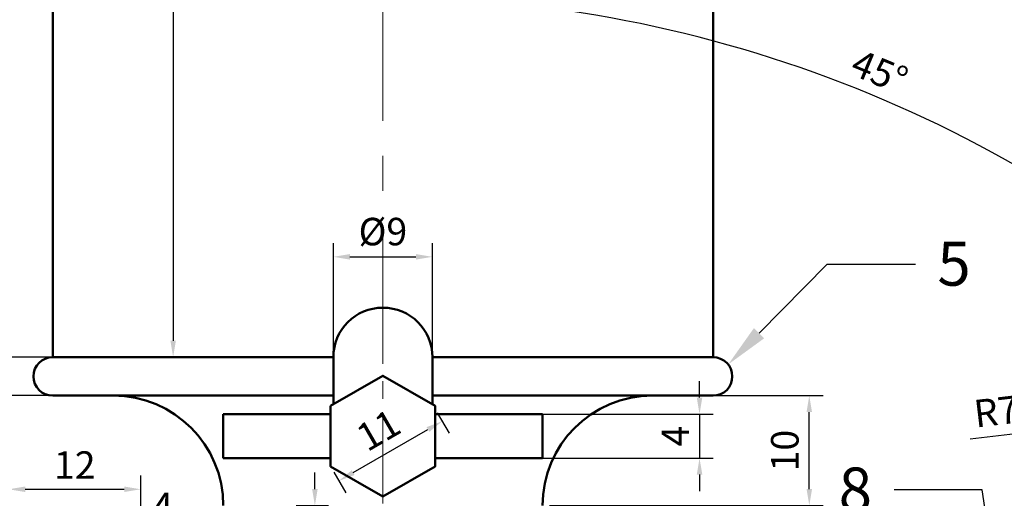
# Model space of a CAD drawing. Units: millimetres. Extents: x -414 to 17, y 81 to 417.
# Tile 4 of 7: x -341 to -252, y 214 to 257. Entities that reach past the tile are written whole.
import ezdxf
from ezdxf import colors
from ezdxf.entities.mleader import LeaderData, LeaderLine
from ezdxf.math import Vec2, Vec3

# ---------------------------------------------------------------- set-up
doc = ezdxf.new("R2010")
doc.units = ezdxf.units.MM
doc.header["$LTSCALE"] = 0.5
doc.linetypes.add('CENTER', pattern=[50.8, 31.75, -6.35, 6.35, -6.35])
for name, color, linetype, lineweight in [('M-CNTR', 1, 'CENTER', 18), ('M-DIMS', 2, 'Continuous', 25), ('M-OUTL', 7, 'Continuous', 50)]:
    doc.layers.add(name, color=color, linetype=linetype, lineweight=lineweight)
doc.styles.get("Standard").update_dxf_attribs({"font": 'arial.ttf'})
doc.dimstyles.new('ISO-25', dxfattribs={"dimtxt": 2.5, "dimasz": 1.5, "dimexe": 1.25, "dimexo": 0.625, "dimtad": 1, "dimtoh": 1, "dimdec": 0, "dimtxsty": 'Standard', "dimcen": 2.5, "dimadec": 0, "dimazin": 0, "dimtfac": 1, "dimtdec": 0, "dimtmove": 0, "dimatfit": 3, "dimfxl": 1, "dimarcsym": 0})

# ---------------------------------------------------------------- blocks, each defined once
blk = doc.blocks.new('*D18')
at = {"layer": 'Defpoints', "color": 0, "ltscale": 0.5, "transparency": 16777216}
for p in [(-328.257, 299.461), (-328.257, 226.461), (-327.548, 226.461)]:
    blk.add_point(p, dxfattribs=at)
at = {"layer": 'M-DIMS', "color": 0, "lineweight": -2, "ltscale": 0.5, "transparency": 16777216}
for p, q in [((-327.632, 299.461), (-326.298, 299.461)), ((-327.548, 297.961), (-327.548, 227.961)), ((-327.632, 226.461), (-326.298, 226.461))]:
    blk.add_line(p, q, dxfattribs=at)
at = {"layer": 'M-DIMS', "color": 0, "ltscale": 0.5, "transparency": 16777216}
for points in [[(-327.798, 297.961), (-327.298, 297.961), (-327.548, 299.461)], [(-327.798, 227.961), (-327.298, 227.961), (-327.548, 226.461)]]:
    blk.add_solid(points, dxfattribs=at)
at = {"layer": 'M-DIMS', "color": 0, "ltscale": 0.5, "transparency": 16777216, "insert": (-329.45, 262.961), "char_height": 2.5, "attachment_point": 5, "rotation": 90}
blk.add_mtext('73', dxfattribs=at)
blk = doc.blocks.new('*D19')
at = {"layer": 'Defpoints', "color": 0, "ltscale": 0.5, "transparency": 16777216}
for p in [(-303.993, 235.587), (-312.993, 226.461), (-303.993, 226.461)]:
    blk.add_point(p, dxfattribs=at)
at = {"layer": 'M-DIMS', "color": 0, "lineweight": -2, "ltscale": 0.5, "transparency": 16777216}
for p, q in [((-312.993, 227.086), (-312.993, 236.837)), ((-303.993, 227.086), (-303.993, 236.837)), ((-311.493, 235.587), (-305.493, 235.587))]:
    blk.add_line(p, q, dxfattribs=at)
at = {"layer": 'M-DIMS', "color": 0, "ltscale": 0.5, "transparency": 16777216}
for points in [[(-311.493, 235.837), (-311.493, 235.337), (-312.993, 235.587)], [(-305.493, 235.837), (-305.493, 235.337), (-303.993, 235.587)]]:
    blk.add_solid(points, dxfattribs=at)
at = {"layer": 'M-DIMS', "color": 0, "ltscale": 0.5, "transparency": 16777216, "insert": (-308.493, 237.559), "char_height": 2.5, "attachment_point": 5}
blk.add_mtext('%%C9', dxfattribs=at)
blk = doc.blocks.new('*D20')
at = {"layer": 'Defpoints', "color": 0, "ltscale": 0.5, "transparency": 16777216}
for p in [(-281.414, 222.961), (-269.748, 222.961), (-293.993, 212.961)]:
    blk.add_point(p, dxfattribs=at)
at = {"layer": 'M-DIMS', "color": 0, "lineweight": -2, "ltscale": 0.5, "transparency": 16777216}
for p, q in [((-280.789, 222.961), (-268.498, 222.961)), ((-269.748, 214.461), (-269.748, 221.461)), ((-293.368, 212.961), (-268.498, 212.961))]:
    blk.add_line(p, q, dxfattribs=at)
at = {"layer": 'M-DIMS', "color": 0, "ltscale": 0.5, "transparency": 16777216}
for points in [[(-269.998, 221.461), (-269.498, 221.461), (-269.748, 222.961)], [(-269.998, 214.461), (-269.498, 214.461), (-269.748, 212.961)]]:
    blk.add_solid(points, dxfattribs=at)
at = {"layer": 'M-DIMS', "color": 0, "ltscale": 0.5, "transparency": 16777216, "insert": (-271.649, 217.961), "char_height": 2.5, "attachment_point": 5, "rotation": 90}
blk.add_mtext('10', dxfattribs=at)
blk = doc.blocks.new('*D21')
at = {"layer": 'Defpoints', "color": 0, "ltscale": 0.5, "transparency": 16777216}
for p in [(-297.507, 221.278), (-297.507, 217.278), (-279.72, 217.278)]:
    blk.add_point(p, dxfattribs=at)
at = {"layer": 'M-DIMS', "color": 0, "lineweight": -2, "ltscale": 0.5, "transparency": 16777216}
for p, q in [((-279.72, 222.778), (-279.72, 224.278)), ((-296.882, 221.278), (-278.47, 221.278)), ((-279.72, 221.278), (-279.72, 217.278)), ((-296.882, 217.278), (-278.47, 217.278)), ((-279.72, 215.778), (-279.72, 214.278))]:
    blk.add_line(p, q, dxfattribs=at)
at = {"layer": 'M-DIMS', "color": 0, "ltscale": 0.5, "transparency": 16777216}
for points in [[(-279.97, 222.778), (-279.47, 222.778), (-279.72, 221.278)], [(-279.97, 215.778), (-279.47, 215.778), (-279.72, 217.278)]]:
    blk.add_solid(points, dxfattribs=at)
at = {"layer": 'M-DIMS', "color": 0, "ltscale": 0.5, "transparency": 16777216, "insert": (-281.595, 219.278), "char_height": 2.5, "attachment_point": 5, "rotation": 90}
blk.add_mtext('4', dxfattribs=at)
blk = doc.blocks.new('*D22')
at = {"layer": 'Defpoints', "color": 0, "ltscale": 0.5, "transparency": 16777216}
for p in [(-303.861, 221.952), (-303.099, 220.632), (-313.256, 216.528)]:
    blk.add_point(p, dxfattribs=at)
at = {"layer": 'M-DIMS', "color": 0, "lineweight": -2, "ltscale": 0.5, "transparency": 16777216}
for p, q in [((-303.549, 221.41), (-302.474, 219.55)), ((-311.195, 215.958), (-304.398, 219.882)), ((-312.943, 215.986), (-311.869, 214.126))]:
    blk.add_line(p, q, dxfattribs=at)
at = {"layer": 'M-DIMS', "color": 0, "ltscale": 0.5, "transparency": 16777216}
for points in [[(-304.523, 220.099), (-304.273, 219.666), (-303.099, 220.632)], [(-311.32, 216.175), (-311.07, 215.742), (-312.494, 215.208)]]:
    blk.add_solid(points, dxfattribs=at)
at = {"layer": 'M-DIMS', "color": 0, "ltscale": 0.5, "transparency": 16777216, "insert": (-308.737, 219.548), "char_height": 2.5, "attachment_point": 5, "rotation": 30}
blk.add_mtext('11', dxfattribs=at)
blk = doc.blocks.new('*D24')
at = {"layer": 'Defpoints', "color": 0, "ltscale": 0.5, "transparency": 16777216}
for p in [(-316.993, 212.961), (-314.671, 212.961), (-316.993, 208.961)]:
    blk.add_point(p, dxfattribs=at)
at = {"layer": 'M-DIMS', "color": 0, "lineweight": -2, "ltscale": 0.5, "transparency": 16777216}
for p, q in [((-314.671, 214.461), (-314.671, 215.961)), ((-316.368, 212.961), (-313.421, 212.961)), ((-314.671, 208.961), (-314.671, 212.961)), ((-316.368, 208.961), (-313.421, 208.961)), ((-314.671, 207.461), (-314.671, 205.961))]:
    blk.add_line(p, q, dxfattribs=at)
at = {"layer": 'M-DIMS', "color": 0, "ltscale": 0.5, "transparency": 16777216}
for points in [[(-314.921, 214.461), (-314.421, 214.461), (-314.671, 212.961)], [(-314.921, 207.461), (-314.421, 207.461), (-314.671, 208.961)]]:
    blk.add_solid(points, dxfattribs=at)
at = {"layer": 'M-DIMS', "color": 0, "ltscale": 0.5, "transparency": 16777216, "insert": (-316.546, 210.961), "char_height": 2.5, "attachment_point": 5, "rotation": 90}
blk.add_mtext('4', dxfattribs=at)
blk = doc.blocks.new('*D29')
at = {"layer": 'Defpoints', "color": 0, "ltscale": 0.5, "transparency": 16777216}
for p in [(-326.493, 210.694), (-330.493, 205.961), (-326.493, 205.961)]:
    blk.add_point(p, dxfattribs=at)
at = {"layer": 'M-DIMS', "color": 0, "lineweight": -2, "ltscale": 0.5, "transparency": 16777216}
for p, q in [((-330.493, 206.586), (-330.493, 211.944)), ((-326.493, 206.586), (-326.493, 211.944)), ((-331.993, 210.694), (-333.493, 210.694)), ((-330.493, 210.694), (-326.493, 210.694)), ((-324.993, 210.694), (-323.493, 210.694))]:
    blk.add_line(p, q, dxfattribs=at)
at = {"layer": 'M-DIMS', "color": 0, "ltscale": 0.5, "transparency": 16777216}
for points in [[(-331.993, 210.944), (-331.993, 210.444), (-330.493, 210.694)], [(-324.993, 210.944), (-324.993, 210.444), (-326.493, 210.694)]]:
    blk.add_solid(points, dxfattribs=at)
at = {"layer": 'M-DIMS', "color": 0, "ltscale": 0.5, "transparency": 16777216, "insert": (-328.493, 212.569), "char_height": 2.5, "attachment_point": 5}
blk.add_mtext('4', dxfattribs=at)
blk = doc.blocks.new('*D30')
at = {"layer": 'Defpoints', "color": 0, "ltscale": 0.5, "transparency": 16777216}
for p in [(-330.493, 214.444), (-330.493, 209.265), (-342.493, 205.101)]:
    blk.add_point(p, dxfattribs=at)
at = {"layer": 'M-DIMS', "color": 0, "lineweight": -2, "ltscale": 0.5, "transparency": 16777216}
for p, q in [((-342.493, 205.726), (-342.493, 215.694)), ((-330.493, 209.89), (-330.493, 215.694)), ((-340.993, 214.444), (-331.993, 214.444))]:
    blk.add_line(p, q, dxfattribs=at)
at = {"layer": 'M-DIMS', "color": 0, "ltscale": 0.5, "transparency": 16777216}
for points in [[(-340.993, 214.694), (-340.993, 214.194), (-342.493, 214.444)], [(-331.993, 214.694), (-331.993, 214.194), (-330.493, 214.444)]]:
    blk.add_solid(points, dxfattribs=at)
at = {"layer": 'M-DIMS', "color": 0, "ltscale": 0.5, "transparency": 16777216, "insert": (-336.493, 216.324), "char_height": 2.5, "attachment_point": 5}
blk.add_mtext('12', dxfattribs=at)
blk = doc.blocks.new('*D37')
at = {"layer": 'Defpoints', "color": 0, "ltscale": 0.5, "transparency": 16777216}
for p in [(-338.493, 222.961), (-374.146, 180.961), (-308.493, 180.961)]:
    blk.add_point(p, dxfattribs=at)
at = {"layer": 'M-DIMS', "color": 0, "lineweight": -2, "ltscale": 0.5, "transparency": 16777216}
for p, q in [((-339.118, 222.961), (-375.396, 222.961)), ((-374.146, 221.461), (-374.146, 182.461)), ((-309.118, 180.961), (-375.396, 180.961))]:
    blk.add_line(p, q, dxfattribs=at)
at = {"layer": 'M-DIMS', "color": 0, "ltscale": 0.5, "transparency": 16777216}
for points in [[(-374.396, 221.461), (-373.896, 221.461), (-374.146, 222.961)], [(-374.396, 182.461), (-373.896, 182.461), (-374.146, 180.961)]]:
    blk.add_solid(points, dxfattribs=at)
at = {"layer": 'M-DIMS', "color": 0, "ltscale": 0.5, "transparency": 16777216, "insert": (-376.027, 201.961), "char_height": 2.5, "attachment_point": 5, "rotation": 90}
blk.add_mtext('42', dxfattribs=at)
blk = doc.blocks.new('*D38')
at = {"layer": 'Defpoints', "color": 0, "ltscale": 0.5, "transparency": 16777216}
for p in [(-333.775, 226.461), (-374.144, 222.961), (-333.775, 222.961)]:
    blk.add_point(p, dxfattribs=at)
at = {"layer": 'M-DIMS', "color": 0, "lineweight": -2, "ltscale": 0.5, "transparency": 16777216}
for p, q in [((-374.144, 227.961), (-374.144, 229.461)), ((-334.4, 226.461), (-375.394, 226.461)), ((-374.144, 226.461), (-374.144, 222.961)), ((-334.4, 222.961), (-375.394, 222.961)), ((-374.144, 221.461), (-374.144, 219.961))]:
    blk.add_line(p, q, dxfattribs=at)
at = {"layer": 'M-DIMS', "color": 0, "ltscale": 0.5, "transparency": 16777216}
for points in [[(-374.394, 227.961), (-373.894, 227.961), (-374.144, 226.461)], [(-374.394, 221.461), (-373.894, 221.461), (-374.144, 222.961)]]:
    blk.add_solid(points, dxfattribs=at)
at = {"layer": 'M-DIMS', "color": 0, "ltscale": 0.5, "transparency": 16777216, "insert": (-376.019, 224.711), "char_height": 2.5, "attachment_point": 5, "rotation": 90}
blk.add_mtext('4', dxfattribs=at)
blk = doc.blocks.new('*D39')
at = {"layer": 'Defpoints', "color": 0, "ltscale": 0.5, "transparency": 16777216}
for p in [(-374.144, 356.468), (-308.493, 356.468), (-361.114, 226.461)]:
    blk.add_point(p, dxfattribs=at)
at = {"layer": 'M-DIMS', "color": 0, "lineweight": -2, "ltscale": 0.5, "transparency": 16777216}
for p, q in [((-309.118, 356.468), (-375.394, 356.468)), ((-374.144, 227.961), (-374.144, 354.968)), ((-361.739, 226.461), (-375.394, 226.461))]:
    blk.add_line(p, q, dxfattribs=at)
at = {"layer": 'M-DIMS', "color": 0, "ltscale": 0.5, "transparency": 16777216}
for points in [[(-374.394, 354.968), (-373.894, 354.968), (-374.144, 356.468)], [(-374.394, 227.961), (-373.894, 227.961), (-374.144, 226.461)]]:
    blk.add_solid(points, dxfattribs=at)
at = {"layer": 'M-DIMS', "color": 0, "ltscale": 0.5, "transparency": 16777216, "insert": (-376.046, 291.464), "char_height": 2.5, "attachment_point": 5, "rotation": 90}
blk.add_mtext('130', dxfattribs=at)
blk = doc.blocks.new('*D57')
at = {"layer": 'Defpoints', "color": 0, "ltscale": 0.5, "transparency": 16777216}
for p in [(-253.851, 219.187), (-246.899, 220.007)]:
    blk.add_point(p, dxfattribs=at)
at = {"layer": 'M-DIMS', "color": 0, "lineweight": -2, "ltscale": 0.5, "transparency": 16777216}
blk.add_line((-255.124, 219.036), (-248.389, 219.831), dxfattribs=at)
at = {"layer": 'M-DIMS', "color": 0, "ltscale": 0.5, "transparency": 16777216}
blk.add_solid([(-248.418, 220.079), (-248.36, 219.583), (-246.899, 220.007)], dxfattribs=at)
at = {"layer": 'M-DIMS', "color": 0, "ltscale": 0.5, "transparency": 16777216, "insert": (-252.721, 221.208), "char_height": 2.5, "attachment_point": 5, "rotation": 6.72795}
blk.add_mtext('R7', dxfattribs=at)
blk = doc.blocks.new('*D70')
at = {"layer": 'Defpoints', "color": 0, "ltscale": 0.5, "transparency": 16777216}
for p in [(-222.226, 229.728), (-308.493, 143.461), (-278.374, 113.343)]:
    blk.add_point(p, dxfattribs=at)
at = {"layer": 'M-DIMS', "color": 0, "lineweight": -2, "ltscale": 0.5, "transparency": 16777216}
for p, q in [((-221.784, 229.286), (-191.223, 198.726)), ((-193.168, 198.549), (-277.314, 114.404)), ((-308.051, 143.019), (-277.49, 112.459))]:
    blk.add_line(p, q, dxfattribs=at)
at = {"layer": 'M-DIMS', "color": 0, "ltscale": 0.5, "transparency": 16777216}
for points in [[(-193.345, 198.726), (-192.991, 198.373), (-192.107, 199.61)], [(-277.49, 114.58), (-277.137, 114.227), (-278.374, 113.343)]]:
    blk.add_solid(points, dxfattribs=at)
at = {"layer": 'M-DIMS', "color": 0, "ltscale": 0.5, "transparency": 16777216, "insert": (-236.57, 157.806), "char_height": 2.5, "attachment_point": 5, "rotation": 45}
blk.add_mtext('122', dxfattribs=at)
blk = doc.blocks.new('*D78')
at = {"layer": 'Defpoints', "color": 0, "ltscale": 0.5, "transparency": 16777216}
for p in [(-308.493, 365.429), (-250.629, 243.684), (-212.22, 239.734), (-308.493, 230.961), (-308.493, 143.461)]:
    blk.add_point(p, dxfattribs=at)
at = {"layer": 'M-DIMS', "color": 0, "lineweight": -2, "ltscale": 0.5, "transparency": 16777216}
blk.add_arc((-308.493, 143.461), 115.727, 45.74265, 89.25735, dxfattribs=at)
at = {"layer": 'M-DIMS', "color": 0, "ltscale": 0.5, "transparency": 16777216}
for points in [[(-306.994, 258.928), (-306.991, 259.428), (-308.493, 259.188)], [(-227.553, 226.524), (-227.905, 226.168), (-226.662, 225.292)]]:
    blk.add_solid(points, dxfattribs=at)
at = {"layer": 'M-DIMS', "color": 0, "ltscale": 0.5, "transparency": 16777216, "insert": (-263.48, 252.131), "char_height": 2.5, "attachment_point": 5, "rotation": 337.5}
blk.add_mtext('45°', dxfattribs=at)

msp = doc.modelspace()

# ---------------------------------------------------------------- linework, layer by layer
at = {"layer": 'M-CNTR'}
msp.add_line((-308.493, 365.429), (-308.493, 230.961), dxfattribs=at)
at = {"layer": 'M-CNTR', "ltscale": 0.5}
msp.add_line((-308.493, 200.461), (-308.493, 230.961), dxfattribs=at)
at = {"layer": 'M-OUTL'}
for p, q in [((-338.493, 299.461), (-338.493, 226.461)), ((-278.493, 299.461), (-278.493, 226.461)), ((-338.493, 226.461), (-312.993, 226.461)), ((-303.993, 226.461), (-278.493, 226.461)), ((-338.493, 222.961), (-312.993, 222.961)), ((-303.993, 222.961), (-278.493, 222.961))]:
    msp.add_line(p, q, dxfattribs=at)
at = {"layer": 'M-OUTL', "ltscale": 0.5}
for p, q in [((-312.993, 226.461), (-312.993, 222.18)), ((-303.993, 226.461), (-303.993, 222.18)), ((-313.256, 221.278), (-322.993, 221.278)), ((-322.993, 221.278), (-322.993, 217.278)), ((-303.73, 221.278), (-293.993, 221.278)), ((-293.993, 221.278), (-293.993, 217.278)), ((-313.256, 217.278), (-322.993, 217.278)), ((-303.73, 217.278), (-293.993, 217.278))]:
    msp.add_line(p, q, dxfattribs=at)
msp.add_lwpolyline([(-313.256, 222.028), (-313.256, 216.528), (-308.493, 213.778), (-303.73, 216.528), (-303.73, 222.028), (-308.493, 224.778)], close=True, dxfattribs=at)
for centre, radius, start, end in [((-308.493, 226.461), 4.5, 0, 180), ((-338.493, 224.711), 1.75, 90, 270), ((-278.493, 224.711), 1.75, 270, 90)]:
    msp.add_arc(centre, radius, start, end, dxfattribs=at)
at = {"layer": 'M-OUTL'}
for centre, start, end in [((-332.993, 212.961), 0, 90), ((-283.993, 212.961), 90, 180)]:
    msp.add_arc(centre, 10, start, end, dxfattribs=at)

# ---------------------------------------------------------------- dimensions: what is measured, and where the dimension line sits
at = {"layer": 'M-DIMS', "ltscale": 0.5}
dim = msp.add_angular_dim_2l(base=(-250.629, 243.684), line1=((-308.493, 365.429), (-308.493, 230.961)), line2=((-212.22, 239.734), (-308.493, 143.461)), dimstyle='ISO-25', override={"dimclrd": 0, "dimclre": 0, "dimclrt": 0}, dxfattribs=at)
dim.commit()
dim.dimension.update_dxf_attribs({"geometry": '*D78', "text_midpoint": (-263.48, 252.131)})
for base, p1, p2, picture, middle in [((-374.144, 356.468), (-361.114, 226.461), (-308.493, 356.468), '*D39', (-376.046, 291.464)), ((-327.548, 226.461), (-328.257, 299.461), (-328.257, 226.461), '*D18', (-329.45, 262.961)), ((-374.144093874, 222.961264832), (-333.77523436, 226.461264832), (-333.77523436, 222.961264832), '*D38', (-376.019093874, 224.711264832)), ((-279.72, 217.278), (-297.507, 221.278), (-297.507, 217.278), '*D21', (-281.595, 219.278)), ((-374.146, 180.961), (-338.493, 222.961), (-308.493, 180.961), '*D37', (-376.027, 201.961)), ((-314.671, 212.961), (-316.993, 208.961), (-316.993, 212.961), '*D24', (-316.546, 210.961))]:
    dim = msp.add_linear_dim(base=base, p1=p1, p2=p2, angle=90, dimstyle='ISO-25', override={"dimclrd": 0, "dimclre": 0, "dimclrt": 0}, dxfattribs=at)
    dim.commit()
    dim.dimension.update_dxf_attribs({"geometry": picture, "text_midpoint": middle})
dim = msp.add_linear_dim(base=(-303.993, 235.587), p1=(-312.993, 226.461), p2=(-303.993, 226.461), text='%%C<>', dimstyle='ISO-25', override={"dimclrd": 0, "dimclre": 0, "dimclrt": 0}, dxfattribs=at)
dim.commit()
dim.dimension.update_dxf_attribs({"geometry": '*D19', "text_midpoint": (-308.493, 237.559)})
for p1, p2, distance, picture, middle in [((-222.226, 229.728), (-308.493, 143.461), 42.594, '*D70', (-236.57, 157.806)), ((-313.256, 216.528), (-303.861, 221.952), -1.524, '*D22', (-308.737, 219.548))]:
    dim = msp.add_aligned_dim(p1=p1, p2=p2, distance=distance, dimstyle='ISO-25', override={"dimclrd": 0, "dimclre": 0, "dimclrt": 0}, dxfattribs=at)
    dim.commit()
    dim.dimension.update_dxf_attribs({"geometry": picture, "text_midpoint": middle})
dim = msp.add_linear_dim(base=(-269.748, 222.961), p1=(-293.993, 212.961), p2=(-281.414, 222.961), angle=90, dimstyle='ISO-25', override={"dimclrd": 0, "dimclre": 0, "dimclrt": 0}, dxfattribs=at)
dim.commit()
dim.dimension.update_dxf_attribs({"geometry": '*D20', "text_midpoint": (-269.748, 217.961), "dimtype": 160})
dim = msp.add_radius_dim(center=(-253.851, 219.187), mpoint=(-246.899, 220.007), dimstyle='ISO-25', override={"dimclrd": 0, "dimclre": 0, "dimclrt": 0}, dxfattribs=at)
dim.commit()
dim.dimension.update_dxf_attribs({"geometry": '*D57', "text_midpoint": (-252.501, 219.346), "dimtype": 164})
for base, p1, p2, picture, middle in [((-330.493, 214.444), (-342.493, 205.101), (-330.493, 209.265), '*D30', (-336.493, 216.324)), ((-326.493, 210.694), (-330.493, 205.961), (-326.493, 205.961), '*D29', (-328.493, 212.569))]:
    dim = msp.add_linear_dim(base=base, p1=p1, p2=p2, dimstyle='ISO-25', override={"dimclrd": 0, "dimclre": 0, "dimclrt": 0}, dxfattribs=at)
    dim.commit()
    dim.dimension.update_dxf_attribs({"geometry": picture, "text_midpoint": middle})

# ---------------------------------------------------------------- leaders
ml = msp.add_multileader_mtext('Standard', dxfattribs=at)
ml.set_content('5', color=256)
ml.set_leader_properties()
ml.build(insert=Vec2(0, 0))
ctx = ml.context
ctx.base_point, ctx.plane_origin = Vec3(-260.112, 234.928), Vec3(-277.119, 225.796)
notes = []
notes.append((ctx, [(0, (1, 1, 0), (-268.112, 234.928), (1, 0), 8, [(0, [(-277.119, 225.796)], 0, [])])]))
ctx.mtext.insert, ctx.mtext.flow_direction = Vec3(-258.112, 236.962), 5
ml = msp.add_multileader_mtext('Standard', dxfattribs=at)
ml.set_content('8', color=256)
ml.set_leader_properties()
ml.build(insert=Vec2(0, 0))
ctx = ml.context
ctx.base_point, ctx.plane_origin = Vec3(-268.685, 214.391), Vec3(-252.631, 204.98)
ctx.text_align_type = 2
notes.append((ctx, [(0, (1, 1, 0), (-254.049, 214.391), (-1, 0), 8, [(0, [(-252.631, 204.98)], 0, [])])]))
ctx.mtext.insert, ctx.mtext.alignment, ctx.mtext.flow_direction = Vec3(-264.049, 216.425), 3, 5
for ctx, leaders in notes:
    for number, flags, end, landing, length, lines in leaders:
        leader = LeaderData()
        leader.index, (leader.has_last_leader_line, leader.has_dogleg_vector, leader.attachment_direction) = number, flags
        leader.last_leader_point, leader.dogleg_vector, leader.dogleg_length = Vec3(end), Vec3(landing), length
        for number, points, colour, breaks in lines:
            line = LeaderLine()
            line.index, line.vertices, line.color, line.breaks = number, Vec3.list(points), colors.encode_raw_color(colour), breaks
            leader.lines.append(line)
        ctx.leaders.append(leader)

doc.saveas('drawing.dxf')
